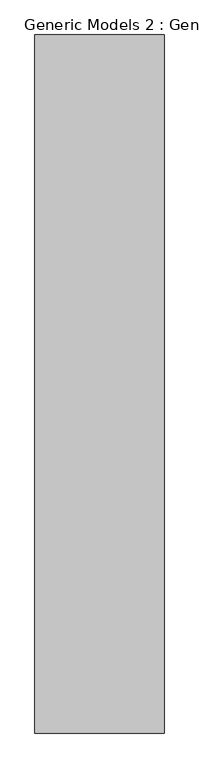
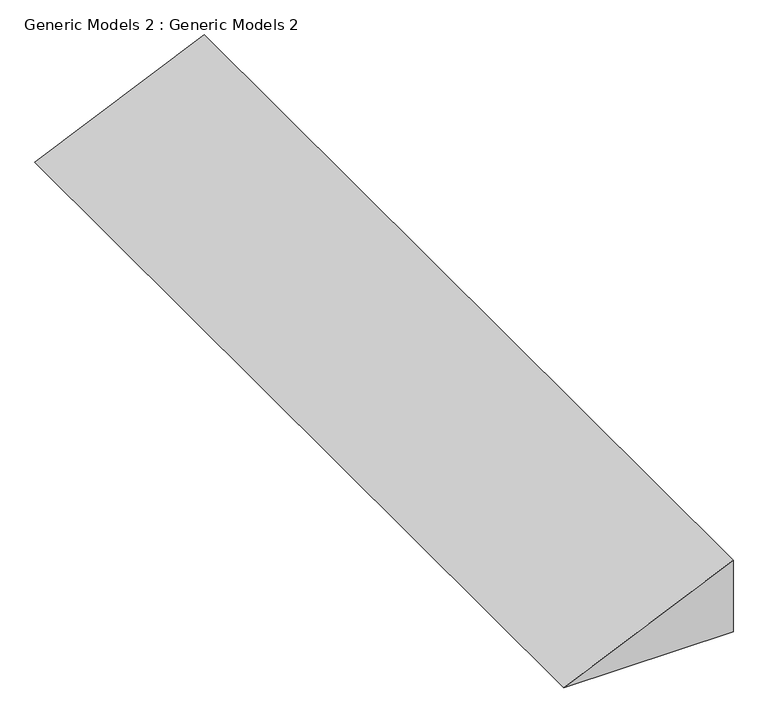
"""IFC4 building model written with IfcOpenShell, lengths in millimetres: proxy geometry, Generic Models 2 : Generic Models 2."""

from ifc_helpers import new_model, si_unit, frame, origin, place, context, project, spatial, polyline, outline, extrude, source, transform, mapped, element, save


def generic_models_2_generic_models_2_939c1542(model_context):
    return source(origin(), model_context, "Body", "SweptSolid", [
        extrude(outline(polyline([(363.0191128, -20862.187975), (0.0, -21677.5422521), (0.0, -20862.187975), (363.0191128, -20862.187975)])), frame((0.0, -2018.2606315, 0.0), z_axis=(0.0, 1.0, 0.0), x_axis=(0.0, 0.0, 1.0)), (0.0, 0.0, 1.0), 4407.1582188),
    ])


if __name__ == "__main__":
    model = new_model("IFC4")
    model_context = context("Model", 3, world=origin())
    ifc_project = project(units=[si_unit("LENGTHUNIT", "METRE", prefix="MILLI")], contexts=[model_context])
    site = spatial("IfcSite", under=ifc_project)
    building = spatial("IfcBuilding", under=site)
    placement = place(None, origin())
    generic_models_2_generic_models_2_shape = generic_models_2_generic_models_2_939c1542(model_context)
    element("IfcBuildingElementProxy", 1, Name="Generic Models 2 : Generic Models 2", ObjectType="Generic Models 2 : Generic Models 2", at=placement, inside=building, context=model_context, shape_type="MappedRepresentation", body=[
        mapped(generic_models_2_generic_models_2_shape, transform((0.0, 0.0, 0.0), x_axis=(1.0, 0.0, 0.0), y_axis=(0.0, 1.0, 0.0), z_axis=(0.0, 0.0, 1.0))),
    ])
    save(model, "model.ifc")

# Revit data of these elements
# Element 1 (IfcBuildingElementProxy, "Generic Models 2 : Generic Models 2")
#   Materials on its faces: "Default New Material(1)"
# Materials
#   "Default New Material(1)": class "Generic", colour RGB 120 120 120, transparency 0, Cost = 0
